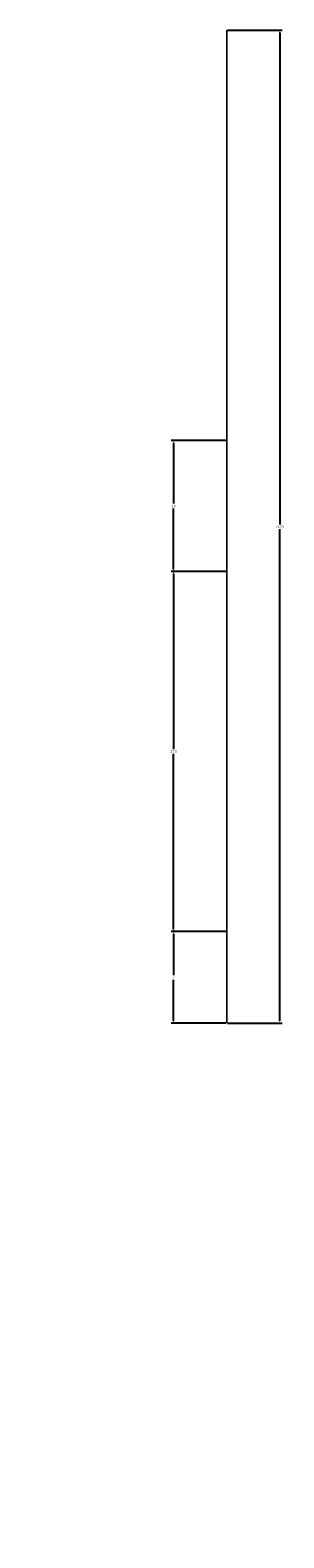
# Model space of a CAD drawing. Units: millimetres. Extents: x -15 to 2550, y 1225 to 3403.
# Tile 1 of 2: x -15 to 4, y 3288 to 3403. Entities that reach past the tile are written whole.
import ezdxf

# ---------------------------------------------------------------- set-up
doc = ezdxf.new("R2010")
doc.units = ezdxf.units.MM
doc.layers.add('M-CONS', color=7, linetype='Continuous', lineweight=18)
doc.layers.add('M-DIMS', color=2, linetype='Continuous', lineweight=18)
doc.styles.get("Standard").update_dxf_attribs({"font": 'arial.ttf'})
doc.dimstyles.get("Standard").update_dxf_attribs({"dimtxt": 0.18, "dimasz": 0.18, "dimexe": 0.18, "dimexo": 0.0625, "dimgap": 0.09, "dimtad": 0, "dimtih": 1, "dimtoh": 1, "dimdec": 4, "dimzin": 0, "dimdsep": 46, "dimtxsty": 'Standard', "dimcen": 0.09, "dimadec": 0, "dimazin": 0, "dimtfac": 1, "dimtdec": 4, "dimtofl": 0, "dimtmove": 0, "dimatfit": 3, "dimfxl": 1, "dimtolj": 1, "dimtzin": 0, "dimarcsym": 0})

# ---------------------------------------------------------------- blocks, each defined once
blk = doc.blocks.new('*D10')
at = {"layer": 'Defpoints', "color": 0, "transparency": 16777216}
for p in [(0, 3403.32), (4.05, 3403.32), (0, 3327.48)]:
    blk.add_point(p, dxfattribs=at)
at = {"layer": 'M-DIMS', "color": 0, "lineweight": -2, "transparency": 16777216}
for p, q in [((0.06, 3403.32), (4.23, 3403.32)), ((4.05, 3403.14), (4.05, 3365.58)), ((4.05, 3327.66), (4.05, 3365.22)), ((0.06, 3327.48), (4.23, 3327.48))]:
    blk.add_line(p, q, dxfattribs=at)
at = {"layer": 'M-DIMS', "color": 0, "transparency": 16777216}
for points in [[(4.02, 3403.14), (4.08, 3403.14), (4.05, 3403.32)], [(4.02, 3327.66), (4.08, 3327.66), (4.05, 3327.48)]]:
    blk.add_solid(points, dxfattribs=at)
at = {"layer": 'M-DIMS', "color": 0, "transparency": 16777216, "insert": (4.05, 3365.4), "char_height": 0.18, "attachment_point": 5}
blk.add_mtext('\\A1;75.83', dxfattribs=at)
blk = doc.blocks.new('*D11')
at = {"layer": 'Defpoints', "color": 0, "transparency": 16777216}
for p in [(-4.05, 3334.484228), (0, 3334.484228), (0, 3327.484228)]:
    blk.add_point(p, dxfattribs=at)
at = {"layer": 'M-DIMS', "color": 0, "lineweight": -2, "transparency": 16777216}
for p, q in [((-0.0625, 3334.484228), (-4.23, 3334.484228)), ((-4.05, 3334.304228), (-4.05, 3331.164228)), ((-4.05, 3327.664228), (-4.05, 3330.804228)), ((-0.0625, 3327.484228), (-4.23, 3327.484228))]:
    blk.add_line(p, q, dxfattribs=at)
at = {"layer": 'M-DIMS', "color": 0, "transparency": 16777216}
for points in [[(-4.08, 3334.304228), (-4.02, 3334.304228), (-4.05, 3334.484228)], [(-4.08, 3327.664228), (-4.02, 3327.664228), (-4.05, 3327.484228)]]:
    blk.add_solid(points, dxfattribs=at)
at = {"layer": 'M-DIMS', "color": 0, "transparency": 16777216, "insert": (-4.05, 3330.984228), "char_height": 0.18, "attachment_point": 5}
blk.add_mtext('\\A1;7', dxfattribs=at)
blk = doc.blocks.new('*D12')
at = {"layer": 'Defpoints', "color": 0, "transparency": 16777216}
for p in [(-4.05, 3361.98), (0, 3361.98), (0, 3334.48)]:
    blk.add_point(p, dxfattribs=at)
at = {"layer": 'M-DIMS', "color": 0, "lineweight": -2, "transparency": 16777216}
for p, q in [((-0.06, 3361.98), (-4.23, 3361.98)), ((-4.05, 3361.8), (-4.05, 3348.42)), ((-4.05, 3334.66), (-4.05, 3348.05)), ((-0.06, 3334.48), (-4.23, 3334.48))]:
    blk.add_line(p, q, dxfattribs=at)
at = {"layer": 'M-DIMS', "color": 0, "transparency": 16777216}
for points in [[(-4.08, 3361.8), (-4.02, 3361.8), (-4.05, 3361.98)], [(-4.08, 3334.66), (-4.02, 3334.66), (-4.05, 3334.48)]]:
    blk.add_solid(points, dxfattribs=at)
at = {"layer": 'M-DIMS', "color": 0, "transparency": 16777216, "insert": (-4.05, 3348.23), "char_height": 0.18, "attachment_point": 5}
blk.add_mtext('\\A1;27.5', dxfattribs=at)
blk = doc.blocks.new('*D13')
at = {"layer": 'Defpoints', "color": 0, "transparency": 16777216}
for p in [(-4.05, 3371.98), (0, 3371.98), (0, 3361.98)]:
    blk.add_point(p, dxfattribs=at)
at = {"layer": 'M-DIMS', "color": 0, "lineweight": -2, "transparency": 16777216}
for p, q in [((-0.06, 3371.98), (-4.23, 3371.98)), ((-4.05, 3371.8), (-4.05, 3367.17)), ((-4.05, 3362.16), (-4.05, 3366.8)), ((-0.06, 3361.98), (-4.23, 3361.98))]:
    blk.add_line(p, q, dxfattribs=at)
at = {"layer": 'M-DIMS', "color": 0, "transparency": 16777216}
for points in [[(-4.08, 3371.8), (-4.02, 3371.8), (-4.05, 3371.98)], [(-4.08, 3362.16), (-4.02, 3362.16), (-4.05, 3361.98)]]:
    blk.add_solid(points, dxfattribs=at)
at = {"layer": 'M-DIMS', "color": 0, "transparency": 16777216, "insert": (-4.05, 3366.98), "char_height": 0.18, "attachment_point": 5}
blk.add_mtext('\\A1;10', dxfattribs=at)

msp = doc.modelspace()

# ---------------------------------------------------------------- linework, layer by layer
at = {"layer": 'M-CONS'}
msp.add_line((-15, 3288.188, -2213.255), (-15, 3288.188, -2220.255), dxfattribs=at)
at = {"layer": 'M-CONS', "extrusion": (1, 0, 0)}
msp.add_lwpolyline([(3366.984, -2227.409, -1), (3366.984, -2196.409), (3403.316, -2196.409, 4.8923745), (3403.316, -2227.409)], format="xyb", close=True, dxfattribs=at)
for centre in [(3366.984, -2184.409), (3366.984, -2239.409), (3339.484, -2211.909)]:
    msp.add_circle(centre, 5, dxfattribs=at)

# ---------------------------------------------------------------- dimensions: what is measured, and where the dimension line sits
at = {"layer": 'M-DIMS'}
for base, p1, p2, override, picture, middle in [((4.05, 3403.316), (0, 3327.484), (0, 3403.316), {"dimdec": 2, "dimlfac": 1, "dimrnd": 0, "dimzin": 0, "dimdsep": 46, "dimlunit": 2}, '*D10', (4.05, 3365.4)), ((-4.05, 3371.984), (0, 3361.984), (0, 3371.984), {"dimdec": 0, "dimlfac": 1, "dimrnd": 0, "dimzin": 0, "dimdsep": 46, "dimlunit": 2}, '*D13', (-4.05, 3366.984)), ((-4.05, 3361.984), (0, 3334.484), (0, 3361.984), {"dimdec": 1, "dimlfac": 1, "dimrnd": 0, "dimzin": 0, "dimdsep": 46, "dimlunit": 2}, '*D12', (-4.05, 3348.234)), ((-4.05, 3334.484), (0, 3327.484), (0, 3334.484), {"dimdec": 0, "dimlfac": 1, "dimrnd": 0, "dimzin": 0, "dimdsep": 46, "dimlunit": 2}, '*D11', (-4.05, 3330.984))]:
    dim = msp.add_linear_dim(base=base, p1=p1, p2=p2, angle=90, dimstyle='Standard', override=override, dxfattribs=at)
    dim.commit()
    dim.dimension.update_dxf_attribs({"geometry": picture, "text_midpoint": middle})

doc.saveas('drawing.dxf')
